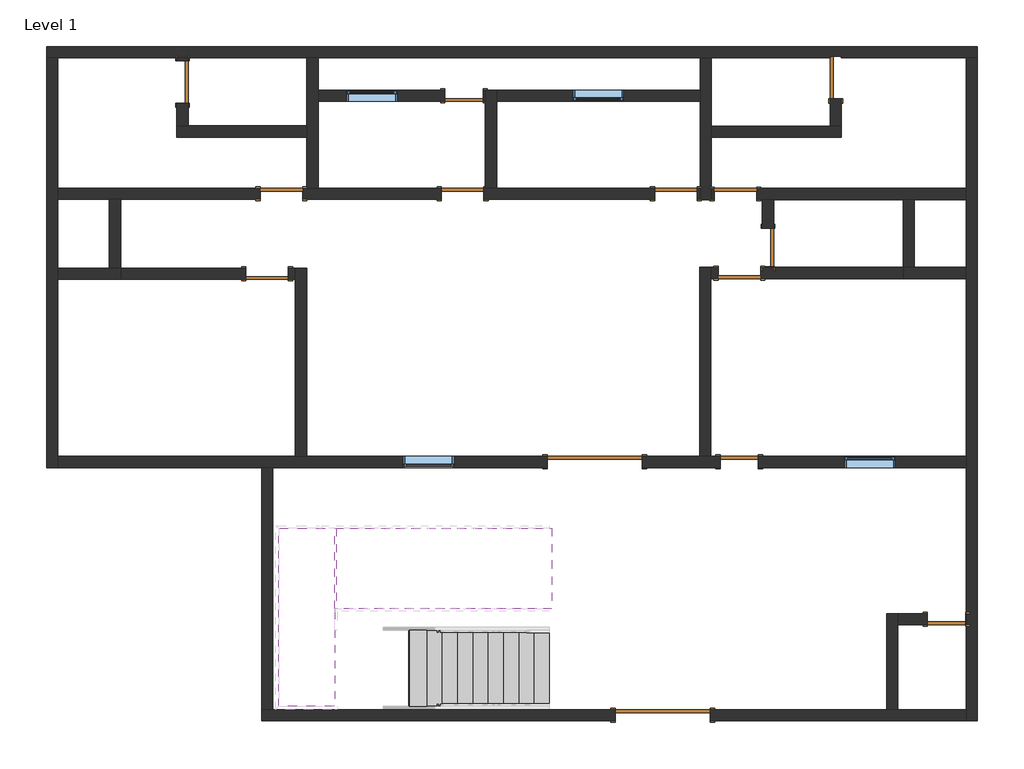
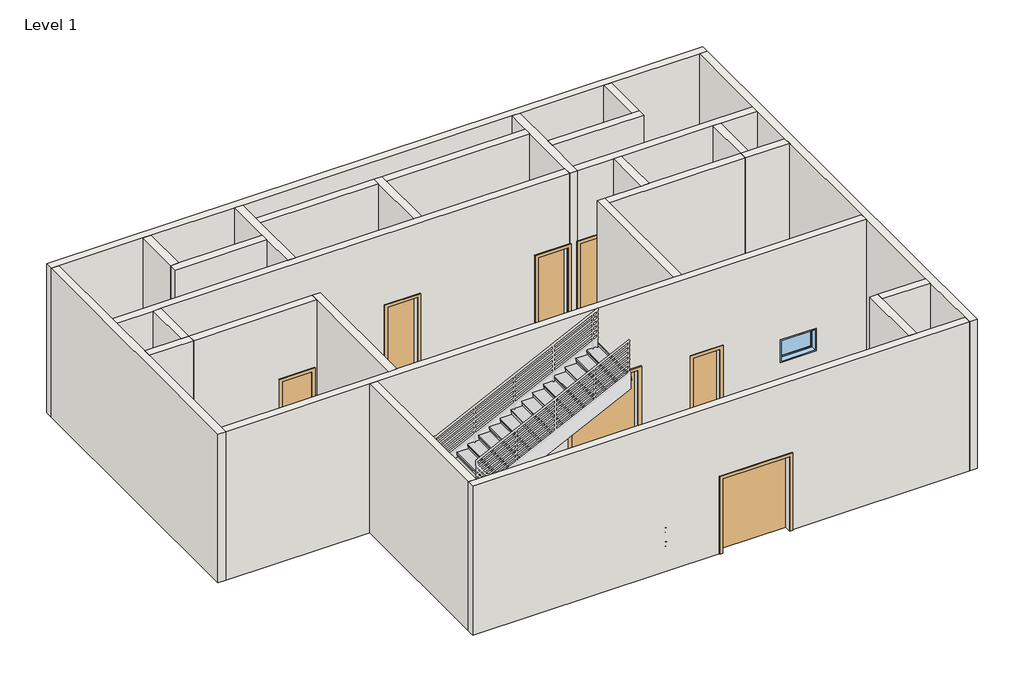
# One storey, part 1 of 4: 28 walls, 14 doors, 4 windows, 2 stair flights, 1 slab.
"""IFC4 building model written with IfcOpenShell, lengths in millimetres."""

from ifc_helpers import new_model, si_unit, frame, origin, origin_with_axes, place, context, project, spatial, polyline, outline, extrude, faceted_brep, transform, mapped, element, save
from components import m_door_double_flush_panel_double_acting_1700_x_2000mm_0a6d9c7f, m_single_flush_0762_x_2032mm_0c256fab, m_single_flush_0762_x_2032mm_7341a4fb, m_single_flush_0762_x_2134mm_f5705a9d, m_single_flush_0762_x_2134mm_85379237, m_single_flush_0762x2022_6401452f, m_single_flush_0762x2022_35973295, non_monolithic_landing_e830aeb0, stair_flight_50mm_tread_25mm_nosing_13mm_riser_e3b9914b, stair_flight_50mm_tread_25mm_nosing_13mm_riser_0c3918f5, m_fixed_0915_x_0610mm_70a843a6

model = new_model("IFC4")

# Units and contexts
model_context = context("Model", 3, world=origin())
ifc_project = project(units=[si_unit("LENGTHUNIT", "METRE", prefix="MILLI")], contexts=[model_context])

# Site, building, storey
site = spatial("IfcSite", under=ifc_project)
building = spatial("IfcBuilding", under=site)
storey = spatial("IfcBuildingStorey", under=building, Name="Level 1", Elevation=0.0)

# Doors
placement = place(None, origin())
m_door_double_flush_panel_double_acting_1700_x_2000mm_shape = m_door_double_flush_panel_double_acting_1700_x_2000mm_0a6d9c7f(model_context)
element("IfcDoor", 1, ObjectType="M_Door-Double-Flush_Panel-Double-Acting : 1700 x 2000mm", at=placement, inside=storey, context=model_context, shape_type="MappedRepresentation", body=[
    mapped(m_door_double_flush_panel_double_acting_1700_x_2000mm_shape, transform((4430.6551601, 3229.9598503, 0.0), x_axis=(1.0, 0.0, 0.0), y_axis=(0.0, 1.0, 0.0), z_axis=(0.0, 0.0, 1.0))),
])
element("IfcDoor", 2, ObjectType="M_Door-Double-Flush_Panel-Double-Acting : 1700 x 2000mm", at=placement, inside=storey, context=model_context, shape_type="MappedRepresentation", body=[
    mapped(m_door_double_flush_panel_double_acting_1700_x_2000mm_shape, transform((5649.8551601, -1313.4901497, 0.0), x_axis=(1.0, 0.0, 0.0), y_axis=(0.0, 1.0, 0.0), z_axis=(0.0, 0.0, 1.0))),
])
m_single_flush_0762_x_2032mm_shape = m_single_flush_0762_x_2032mm_0c256fab(model_context)
element("IfcDoor", 3, ObjectType="M_Single-Flush : 0762 x 2032mm", at=placement, inside=storey, context=model_context, shape_type="MappedRepresentation", body=[
    mapped(m_single_flush_0762_x_2032mm_shape, transform((-1189.0948399, 8036.9098503, 0.0), x_axis=(1.0, 0.0, 0.0), y_axis=(0.0, 1.0, 0.0), z_axis=(0.0, 0.0, 1.0))),
])
element("IfcDoor", 4, ObjectType="M_Single-Flush : 0762 x 2032mm", at=placement, inside=storey, context=model_context, shape_type="MappedRepresentation", body=[
    mapped(m_single_flush_0762_x_2032mm_shape, transform((8750.2551601, 10119.7098503, 0.0), x_axis=(0.0, 1.0, 0.0), y_axis=(-1.0, 0.0, 0.0), z_axis=(0.0, 0.0, 1.0))),
])
element("IfcDoor", 5, ObjectType="M_Single-Flush : 0762 x 2032mm", at=placement, inside=storey, context=model_context, shape_type="MappedRepresentation", body=[
    mapped(m_single_flush_0762_x_2032mm_shape, transform((2062.1051601, 8036.9098503, 0.0), x_axis=(1.0, 0.0, 0.0), y_axis=(0.0, 1.0, 0.0), z_axis=(0.0, 0.0, 1.0))),
])
element("IfcDoor", 6, ObjectType="M_Single-Flush : 0762 x 2032mm", at=placement, inside=storey, context=model_context, shape_type="MappedRepresentation", body=[
    mapped(m_single_flush_0762_x_2032mm_shape, transform((5883.2551601, 8036.9098503, 0.0), x_axis=(1.0, 0.0, 0.0), y_axis=(0.0, 1.0, 0.0), z_axis=(0.0, 0.0, 1.0))),
])
m_single_flush_0762_x_2032mm_2_shape = m_single_flush_0762_x_2032mm_7341a4fb(model_context)
element("IfcDoor", 7, ObjectType="M_Single-Flush : 0762 x 2032mm", at=placement, inside=storey, context=model_context, shape_type="MappedRepresentation", body=[
    mapped(m_single_flush_0762_x_2032mm_2_shape, transform((-2960.7448399, 10043.5098503, 0.0), x_axis=(0.0, 1.0, 0.0), y_axis=(-1.0, 0.0, 0.0), z_axis=(0.0, 0.0, 1.0))),
])
element("IfcDoor", 8, ObjectType="M_Single-Flush : 0762 x 2032mm", at=placement, inside=storey, context=model_context, shape_type="MappedRepresentation", body=[
    mapped(m_single_flush_0762_x_2032mm_2_shape, transform((6950.0551601, 8033.7098503, 0.0), x_axis=(-1.0, 0.0, 0.0), y_axis=(0.0, -1.0, 0.0), z_axis=(0.0, 0.0, 1.0))),
])
m_single_flush_0762_x_2134mm_shape = m_single_flush_0762_x_2134mm_f5705a9d(model_context)
element("IfcDoor", 9, ObjectType="M_Single-Flush : 0762 x 2134mm", at=placement, inside=storey, context=model_context, shape_type="MappedRepresentation", body=[
    mapped(m_single_flush_0762_x_2134mm_shape, transform((-1444.6948399, 6603.4098503, 0.0), x_axis=(1.0, 0.0, 0.0), y_axis=(0.0, 1.0, 0.0), z_axis=(0.0, 0.0, 1.0))),
])
m_single_flush_0762_x_2134mm_2_shape = m_single_flush_0762_x_2134mm_85379237(model_context)
element("IfcDoor", 10, ObjectType="M_Single-Flush : 0762 x 2134mm", at=placement, inside=storey, context=model_context, shape_type="MappedRepresentation", body=[
    mapped(m_single_flush_0762_x_2134mm_2_shape, transform((7021.4551601, 6616.0598503, 0.0), x_axis=(-1.0, 0.0, 0.0), y_axis=(0.0, -1.0, 0.0), z_axis=(0.0, 0.0, 1.0))),
])
m_single_flush_0762x2022_shape = m_single_flush_0762x2022_6401452f(model_context)
element("IfcDoor", 11, ObjectType="M_Single-Flush : 0762X2022", at=placement, inside=storey, context=model_context, shape_type="MappedRepresentation", body=[
    mapped(m_single_flush_0762x2022_shape, transform((2087.5051601, 9792.7098503, 0.0), x_axis=(1.0, 0.0, 0.0), y_axis=(0.0, 1.0, 0.0), z_axis=(0.0, 0.0, 1.0))),
])
element("IfcDoor", 12, ObjectType="M_Single-Flush : 0762X2022", at=placement, inside=storey, context=model_context, shape_type="MappedRepresentation", body=[
    mapped(m_single_flush_0762x2022_shape, transform((10733.0551601, 410.5098503, 0.0), x_axis=(1.0, 0.0, 0.0), y_axis=(0.0, 1.0, 0.0), z_axis=(0.0, 0.0, 1.0))),
])
element("IfcDoor", 13, ObjectType="M_Single-Flush : 0762X2022", at=placement, inside=storey, context=model_context, shape_type="MappedRepresentation", body=[
    mapped(m_single_flush_0762x2022_shape, transform((7021.4551601, 3229.9598503, 0.0), x_axis=(-1.0, 0.0, 0.0), y_axis=(0.0, -1.0, 0.0), z_axis=(0.0, 0.0, 1.0))),
])
m_single_flush_0762x2022_2_shape = m_single_flush_0762x2022_35973295(model_context)
element("IfcDoor", 14, ObjectType="M_Single-Flush : 0762X2022", at=placement, inside=storey, context=model_context, shape_type="MappedRepresentation", body=[
    mapped(m_single_flush_0762x2022_2_shape, transform((7535.8551601, 7073.2598503, 0.0), x_axis=(0.0, -1.0, 0.0), y_axis=(1.0, 0.0, 0.0), z_axis=(0.0, 0.0, 1.0))),
])

# Slab
non_monolithic_landing_shape = non_monolithic_landing_e830aeb0(model_context)
element("IfcSlab", 15, ObjectType="Non-Monolithic Landing", at=placement, inside=storey, context=model_context, shape_type="MappedRepresentation", body=[
    mapped(non_monolithic_landing_shape, transform((0.0, 0.0, 0.0), x_axis=(1.0, 0.0, 0.0), y_axis=(0.0, 1.0, 0.0), z_axis=(0.0, 0.0, 1.0))),
])

# Stair flights
stair_flight_50mm_tread_25mm_nosing_13mm_riser_shape = stair_flight_50mm_tread_25mm_nosing_13mm_riser_e3b9914b(model_context)
element("IfcStairFlight", 16, ObjectType="50mm Tread 25mm Nosing 13mm Riser", at=placement, inside=storey, context=model_context, shape_type="MappedRepresentation", body=[
    mapped(stair_flight_50mm_tread_25mm_nosing_13mm_riser_shape, transform((0.0, 0.0, 0.0), x_axis=(1.0, 0.0, 0.0), y_axis=(0.0, 1.0, 0.0), z_axis=(0.0, 0.0, 1.0))),
])
stair_flight_50mm_tread_25mm_nosing_13mm_riser_2_shape = stair_flight_50mm_tread_25mm_nosing_13mm_riser_0c3918f5(model_context)
element("IfcStairFlight", 17, ObjectType="50mm Tread 25mm Nosing 13mm Riser", at=placement, inside=storey, context=model_context, shape_type="MappedRepresentation", body=[
    mapped(stair_flight_50mm_tread_25mm_nosing_13mm_riser_2_shape, transform((0.0, 0.0, 0.0), x_axis=(1.0, 0.0, 0.0), y_axis=(0.0, 1.0, 0.0), z_axis=(0.0, 0.0, 1.0))),
])

# Walls
element("IfcWall", 18, ObjectType="Generic - 200mm", at=placement, inside=storey, context=model_context, shape_type="Brep", body=[
    faceted_brep([(11290.2551601, 10476.9098503, 4000.0), (11090.2551601, 10476.9098503, 4000.0), (8850.2551601, 10476.9098503, 4000.0), (8650.2551601, 10476.9098503, 4000.0), (6516.6551601, 10476.9098503, 4000.0), (6316.6551601, 10476.9098503, 4000.0), (-530.2948399, 10476.9098503, 4000.0), (-730.2948399, 10476.9098503, 4000.0), (-2860.7448399, 10476.9098503, 4000.0), (-3060.7448399, 10476.9098503, 4000.0), (-5197.5448399, 10476.9098503, 4000.0), (-5397.5448399, 10476.9098503, 4000.0), (-5397.5448399, 10476.9098503, 0.0), (-5197.5448399, 10476.9098503, 0.0), (-3060.7448399, 10476.9098503, 0.0), (-2860.7448399, 10476.9098503, 0.0), (-730.2948399, 10476.9098503, 0.0), (-530.2948399, 10476.9098503, 0.0), (6316.6551601, 10476.9098503, 0.0), (6516.6551601, 10476.9098503, 0.0), (8650.2551601, 10476.9098503, 0.0), (8650.2551601, 10476.9098503, 2032.0), (8850.2551601, 10476.9098503, 2032.0), (8850.2551601, 10476.9098503, 0.0), (11090.2551601, 10476.9098503, 0.0), (11290.2551601, 10476.9098503, 0.0), (11290.2551601, 10676.9098503, 0.0), (-5397.5448399, 10676.9098503, 0.0), (-5397.5448399, 10676.9098503, 4000.0), (11290.2551601, 10676.9098503, 4000.0), (8850.2551601, 10500.7098503, 0.0), (8650.2551601, 10500.7098503, 0.0), (8850.2551601, 10500.7098503, 2032.0), (8650.2551601, 10500.7098503, 2032.0)], [[[0, 1, 2, 3, 4, 5, 6, 7, 8, 9, 10, 11, 12, 13, 14, 15, 16, 17, 18, 19, 20, 21, 22, 23, 24, 25]], [[26, 27, 28, 29]], [[27, 26, 25, 24, 23, 30, 31, 20, 19, 18, 17, 16, 15, 14, 13, 12]], [[11, 10, 9, 8, 7, 6, 5, 4, 3, 2, 1, 0, 29, 28]], [[0, 25, 26, 29]], [[12, 11, 28, 27]], [[32, 30, 23, 22]], [[31, 33, 21, 20]], [[30, 32, 33, 31]], [[33, 32, 22, 21]]]),
])
element("IfcWall", 19, ObjectType="Generic - 200mm", at=placement, inside=storey, context=model_context, shape_type="Brep", body=[
    faceted_brep([(11090.2551601, 10476.9098503, 0.0), (11090.2551601, 8133.7098503, 0.0), (11090.2551601, 7933.7098503, 0.0), (11090.2551601, 6716.0598503, 0.0), (11090.2551601, 6516.0598503, 0.0), (11090.2551601, 3329.9598503, 0.0), (11090.2551601, 3129.9598503, 0.0), (11090.2551601, 510.5098503, 0.0), (11090.2551601, 310.5098503, 0.0), (11090.2551601, -1213.4901497, 0.0), (11090.2551601, -1413.4901497, 0.0), (11090.2551601, -1413.4901497, 4000.0), (11090.2551601, -1213.4901497, 4000.0), (11090.2551601, 310.5098503, 4000.0), (11090.2551601, 510.5098503, 4000.0), (11090.2551601, 3129.9598503, 4000.0), (11090.2551601, 3329.9598503, 4000.0), (11090.2551601, 6516.0598503, 4000.0), (11090.2551601, 6716.0598503, 4000.0), (11090.2551601, 7933.7098503, 4000.0), (11090.2551601, 8133.7098503, 4000.0), (11090.2551601, 10476.9098503, 4000.0), (11290.2551601, 10476.9098503, 0.0), (11290.2551601, 10476.9098503, 4000.0), (11290.2551601, -1413.4901497, 4000.0), (11290.2551601, -1413.4901497, 0.0)], [[[0, 1, 2, 3, 4, 5, 6, 7, 8, 9, 10, 11, 12, 13, 14, 15, 16, 17, 18, 19, 20, 21]], [[22, 23, 24, 25]], [[10, 9, 8, 7, 6, 5, 4, 3, 2, 1, 0, 22, 25]], [[21, 20, 19, 18, 17, 16, 15, 14, 13, 12, 11, 24, 23]], [[0, 21, 23, 22]], [[11, 10, 25, 24]]]),
])
element("IfcWall", 20, ObjectType="Generic - 200mm", at=placement, inside=storey, context=model_context, shape_type="Brep", body=[
    faceted_brep([(-1543.0948399, -1213.4901497, 4000.0), (-1343.0948399, -1213.4901497, 4000.0), (9664.6551601, -1213.4901497, 4000.0), (9864.6551601, -1213.4901497, 4000.0), (11090.2551601, -1213.4901497, 4000.0), (11090.2551601, -1213.4901497, 0.0), (9864.6551601, -1213.4901497, 0.0), (9664.6551601, -1213.4901497, 0.0), (6499.8551601, -1213.4901497, 0.0), (6499.8551601, -1213.4901497, 2000.0), (4799.8551601, -1213.4901497, 2000.0), (4799.8551601, -1213.4901497, 0.0), (-1343.0948399, -1213.4901497, 0.0), (-1543.0948399, -1213.4901497, 0.0), (11090.2551601, -1413.4901497, 4000.0), (-1543.0948399, -1413.4901497, 4000.0), (-1543.0948399, -1413.4901497, 0.0), (4799.8551601, -1413.4901497, 0.0), (4799.8551601, -1413.4901497, 2000.0), (6499.8551601, -1413.4901497, 2000.0), (6499.8551601, -1413.4901497, 0.0), (11090.2551601, -1413.4901497, 0.0)], [[[0, 1, 2, 3, 4, 5, 6, 7, 8, 9, 10, 11, 12, 13]], [[14, 15, 16, 17, 18, 19, 20, 21]], [[5, 21, 20, 8, 7, 6]], [[16, 13, 12, 11, 17]], [[4, 3, 2, 1, 0, 15, 14]], [[5, 4, 14, 21]], [[0, 13, 16, 15]], [[19, 9, 8, 20]], [[9, 19, 18, 10]], [[10, 18, 17, 11]]]),
])
element("IfcWall", 21, ObjectType="Generic - 200mm", at=placement, inside=storey, context=model_context, shape_type="Brep", body=[
    faceted_brep([(-5197.5448399, 3129.9598503, 0.0), (-5197.5448399, 3329.9598503, 0.0), (-5197.5448399, 6503.4098503, 0.0), (-5197.5448399, 6703.4098503, 0.0), (-5197.5448399, 7936.9098503, 0.0), (-5197.5448399, 8136.9098503, 0.0), (-5197.5448399, 10476.9098503, 0.0), (-5197.5448399, 10476.9098503, 4000.0), (-5197.5448399, 8136.9098503, 4000.0), (-5197.5448399, 7936.9098503, 4000.0), (-5197.5448399, 6703.4098503, 4000.0), (-5197.5448399, 6503.4098503, 4000.0), (-5197.5448399, 3329.9598503, 4000.0), (-5197.5448399, 3129.9598503, 4000.0), (-5397.5448399, 3129.9598503, 0.0), (-5397.5448399, 3129.9598503, 4000.0), (-5397.5448399, 10476.9098503, 4000.0), (-5397.5448399, 10476.9098503, 0.0)], [[[0, 1, 2, 3, 4, 5, 6, 7, 8, 9, 10, 11, 12, 13]], [[14, 15, 16, 17]], [[6, 5, 4, 3, 2, 1, 0, 14, 17]], [[13, 12, 11, 10, 9, 8, 7, 16, 15]], [[7, 6, 17, 16]], [[0, 13, 15, 14]]]),
])
element("IfcWall", 22, ObjectType="Generic - 200mm", at=placement, inside=storey, context=model_context, shape_type="Brep", body=[
    faceted_brep([(-530.2948399, 8136.9098503, 0.0), (-530.2948399, 9692.7098503, 0.0), (-530.2948399, 9892.7098503, 0.0), (-530.2948399, 10476.9098503, 0.0), (-530.2948399, 10476.9098503, 4000.0), (-530.2948399, 9892.7098503, 4000.0), (-530.2948399, 9692.7098503, 4000.0), (-530.2948399, 8136.9098503, 4000.0), (-730.2948399, 8136.9098503, 0.0), (-730.2948399, 8136.9098503, 4000.0), (-730.2948399, 9052.9098503, 4000.0), (-730.2948399, 9252.9098503, 4000.0), (-730.2948399, 10476.9098503, 4000.0), (-730.2948399, 10476.9098503, 0.0), (-730.2948399, 9252.9098503, 0.0), (-730.2948399, 9052.9098503, 0.0)], [[[0, 1, 2, 3, 4, 5, 6, 7]], [[8, 9, 10, 11, 12, 13, 14, 15]], [[3, 2, 1, 0, 8, 15, 14, 13]], [[7, 6, 5, 4, 12, 11, 10, 9]], [[4, 3, 13, 12]], [[0, 7, 9, 8]]]),
])
element("IfcWall", 23, ObjectType="Generic - 200mm", at=placement, inside=storey, context=model_context, shape_type="Brep", body=[
    faceted_brep([(6264.2551601, 7936.9098503, 2032.0), (6264.2551601, 7936.9098503, 0.0), (6316.6551601, 7936.9098503, 0.0), (6316.6551601, 7936.9098503, 4000.0), (-4070.4448399, 7936.9098503, 4000.0), (-4270.4448399, 7936.9098503, 4000.0), (-5197.5448399, 7936.9098503, 4000.0), (-5197.5448399, 7936.9098503, 0.0), (-4270.4448399, 7936.9098503, 0.0), (-4070.4448399, 7936.9098503, 0.0), (-1570.0948399, 7936.9098503, 0.0), (-1570.0948399, 7936.9098503, 2032.0), (-808.0948399, 7936.9098503, 2032.0), (-808.0948399, 7936.9098503, 0.0), (1681.1051601, 7936.9098503, 0.0), (1681.1051601, 7936.9098503, 2032.0), (2443.1051601, 7936.9098503, 2032.0), (2443.1051601, 7936.9098503, 0.0), (5502.2551601, 7936.9098503, 0.0), (5502.2551601, 7936.9098503, 2032.0), (6316.6551601, 8136.9098503, 0.0), (6264.2551601, 8136.9098503, 0.0), (6264.2551601, 8136.9098503, 2032.0), (5502.2551601, 8136.9098503, 2032.0), (5502.2551601, 8136.9098503, 0.0), (2670.1051601, 8136.9098503, 0.0), (2470.1051601, 8136.9098503, 0.0), (2443.1051601, 8136.9098503, 0.0), (2443.1051601, 8136.9098503, 2032.0), (1681.1051601, 8136.9098503, 2032.0), (1681.1051601, 8136.9098503, 0.0), (-530.2948399, 8136.9098503, 0.0), (-730.2948399, 8136.9098503, 0.0), (-808.0948399, 8136.9098503, 0.0), (-808.0948399, 8136.9098503, 2032.0), (-1570.0948399, 8136.9098503, 2032.0), (-1570.0948399, 8136.9098503, 0.0), (-5197.5448399, 8136.9098503, 0.0), (-5197.5448399, 8136.9098503, 4000.0), (-730.2948399, 8136.9098503, 4000.0), (-530.2948399, 8136.9098503, 4000.0), (2470.1051601, 8136.9098503, 4000.0), (2670.1051601, 8136.9098503, 4000.0), (6316.6551601, 8136.9098503, 4000.0)], [[[0, 1, 2, 3, 4, 5, 6, 7, 8, 9, 10, 11, 12, 13, 14, 15, 16, 17, 18, 19]], [[20, 21, 22, 23, 24, 25, 26, 27, 28, 29, 30, 31, 32, 33, 34, 35, 36, 37, 38, 39, 40, 41, 42, 43]], [[14, 13, 33, 32, 31, 30]], [[18, 17, 27, 26, 25, 24]], [[2, 1, 21, 20]], [[10, 9, 8, 7, 37, 36]], [[6, 5, 4, 3, 43, 42, 41, 40, 39, 38]], [[7, 6, 38, 37]], [[34, 33, 13, 12]], [[35, 34, 12, 11]], [[36, 35, 11, 10]], [[3, 2, 20, 43]], [[28, 27, 17, 16]], [[29, 28, 16, 15]], [[30, 29, 15, 14]], [[22, 21, 1, 0]], [[23, 22, 0, 19]], [[24, 23, 19, 18]]]),
])
element("IfcWall", 24, ObjectType="Generic - 200mm", at=placement, inside=storey, context=model_context, shape_type="Brep", body=[
    faceted_brep([(-730.2948399, 9252.9098503, 0.0), (-2860.7448399, 9252.9098503, 0.0), (-3060.7448399, 9252.9098503, 0.0), (-3060.7448399, 9252.9098503, 4000.0), (-2860.7448399, 9252.9098503, 4000.0), (-730.2948399, 9252.9098503, 4000.0), (-730.2948399, 9052.9098503, 0.0), (-730.2948399, 9052.9098503, 4000.0), (-3060.7448399, 9052.9098503, 4000.0), (-3060.7448399, 9052.9098503, 0.0)], [[[0, 1, 2, 3, 4, 5]], [[6, 7, 8, 9]], [[2, 1, 0, 6, 9]], [[5, 4, 3, 8, 7]], [[0, 5, 7, 6]], [[3, 2, 9, 8]]]),
])
element("IfcWall", 25, ObjectType="Generic - 200mm", at=placement, inside=storey, context=model_context, shape_type="SweptSolid", body=[
    extrude(outline(polyline([(10476.9098503, 0.0), (10424.5098503, 0.0), (10424.5098503, 2032.0), (9662.5098503, 2032.0), (9662.5098503, 0.0), (9252.9098503, 0.0), (9252.9098503, 4000.0), (10476.9098503, 4000.0), (10476.9098503, 0.0)])), frame((-3060.7448399, 0.0, 0.0), z_axis=(1.0, 0.0, 0.0), x_axis=(0.0, 1.0, 0.0)), (0.0, 0.0, 1.0), 200.0),
])
element("IfcWall", 26, ObjectType="Generic - 200mm", at=placement, inside=storey, context=model_context, shape_type="Brep", body=[
    faceted_brep([(6316.6551601, 10476.9098503, 0.0), (6316.6551601, 9892.7098503, 0.0), (6316.6551601, 9692.7098503, 0.0), (6316.6551601, 8136.9098503, 0.0), (6316.6551601, 7936.9098503, 0.0), (6316.6551601, 7933.7098503, 0.0), (6316.6551601, 7933.7098503, 4000.0), (6316.6551601, 7936.9098503, 4000.0), (6316.6551601, 8136.9098503, 4000.0), (6316.6551601, 9692.7098503, 4000.0), (6316.6551601, 9892.7098503, 4000.0), (6316.6551601, 10476.9098503, 4000.0), (6516.6551601, 10476.9098503, 0.0), (6516.6551601, 10476.9098503, 4000.0), (6516.6551601, 9248.1598503, 4000.0), (6516.6551601, 9048.1598503, 4000.0), (6516.6551601, 8133.7098503, 4000.0), (6516.6551601, 7933.7098503, 4000.0), (6516.6551601, 7933.7098503, 0.0), (6516.6551601, 8133.7098503, 0.0), (6516.6551601, 9048.1598503, 0.0), (6516.6551601, 9248.1598503, 0.0)], [[[0, 1, 2, 3, 4, 5, 6, 7, 8, 9, 10, 11]], [[12, 13, 14, 15, 16, 17, 18, 19, 20, 21]], [[5, 4, 3, 2, 1, 0, 12, 21, 20, 19, 18]], [[11, 10, 9, 8, 7, 6, 17, 16, 15, 14, 13]], [[0, 11, 13, 12]], [[6, 5, 18, 17]]]),
])
element("IfcWall", 27, ObjectType="Generic - 200mm", at=placement, inside=storey, context=model_context, shape_type="Brep", body=[
    faceted_brep([(6516.6551601, 7933.7098503, 0.0), (6569.0551601, 7933.7098503, 0.0), (6569.0551601, 7933.7098503, 2032.0), (7331.0551601, 7933.7098503, 2032.0), (7331.0551601, 7933.7098503, 0.0), (7435.8551601, 7933.7098503, 0.0), (7635.8551601, 7933.7098503, 0.0), (9959.9551601, 7933.7098503, 0.0), (10159.9551601, 7933.7098503, 0.0), (11090.2551601, 7933.7098503, 0.0), (11090.2551601, 7933.7098503, 4000.0), (10159.9551601, 7933.7098503, 4000.0), (9959.9551601, 7933.7098503, 4000.0), (7635.8551601, 7933.7098503, 4000.0), (7435.8551601, 7933.7098503, 4000.0), (6516.6551601, 7933.7098503, 4000.0), (6569.0551601, 8133.7098503, 2032.0), (6569.0551601, 8133.7098503, 0.0), (6516.6551601, 8133.7098503, 0.0), (6516.6551601, 8133.7098503, 4000.0), (11090.2551601, 8133.7098503, 4000.0), (11090.2551601, 8133.7098503, 0.0), (7331.0551601, 8133.7098503, 0.0), (7331.0551601, 8133.7098503, 2032.0)], [[[0, 1, 2, 3, 4, 5, 6, 7, 8, 9, 10, 11, 12, 13, 14, 15]], [[16, 17, 18, 19, 20, 21, 22, 23]], [[22, 21, 9, 8, 7, 6, 5, 4]], [[18, 17, 1, 0]], [[15, 14, 13, 12, 11, 10, 20, 19]], [[0, 15, 19, 18]], [[10, 9, 21, 20]], [[2, 1, 17, 16]], [[3, 2, 16, 23]], [[4, 3, 23, 22]]]),
])
element("IfcWall", 28, ObjectType="Generic - 200mm", at=placement, inside=storey, context=model_context, shape_type="Brep", body=[
    faceted_brep([(6516.6551601, 9048.1598503, 0.0), (8850.2551601, 9048.1598503, 0.0), (8850.2551601, 9048.1598503, 4000.0), (6516.6551601, 9048.1598503, 4000.0), (6516.6551601, 9248.1598503, 0.0), (6516.6551601, 9248.1598503, 4000.0), (8650.2551601, 9248.1598503, 4000.0), (8850.2551601, 9248.1598503, 4000.0), (8850.2551601, 9248.1598503, 0.0), (8650.2551601, 9248.1598503, 0.0)], [[[0, 1, 2, 3]], [[4, 5, 6, 7, 8, 9]], [[1, 0, 4, 9, 8]], [[3, 2, 7, 6, 5]], [[0, 3, 5, 4]], [[2, 1, 8, 7]]]),
])
element("IfcWall", 29, ObjectType="Generic - 200mm", at=placement, inside=storey, context=model_context, shape_type="SweptSolid", body=[
    extrude(outline(polyline([(9248.1598503, 4000.0), (10476.9098503, 4000.0), (10476.9098503, 2032.0), (9738.7098503, 2032.0), (9738.7098503, 0.0), (9248.1598503, 0.0), (9248.1598503, 4000.0)])), frame((8650.2551601, 0.0, 0.0), z_axis=(1.0, 0.0, 0.0), x_axis=(0.0, 1.0, 0.0)), (0.0, 0.0, 1.0), 200.0),
])
element("IfcWall", 30, ObjectType="Generic - 200mm", at=placement, inside=storey, context=model_context, shape_type="Brep", body=[
    faceted_brep([(2670.1051601, 8136.9098503, 0.0), (2670.1051601, 9692.7098503, 0.0), (2670.1051601, 9892.7098503, 0.0), (2670.1051601, 9892.7098503, 4000.0), (2670.1051601, 9692.7098503, 4000.0), (2670.1051601, 8136.9098503, 4000.0), (2470.1051601, 8136.9098503, 0.0), (2470.1051601, 8136.9098503, 4000.0), (2470.1051601, 9692.7098503, 4000.0), (2470.1051601, 9892.7098503, 4000.0), (2470.1051601, 9892.7098503, 0.0), (2470.1051601, 9692.7098503, 0.0)], [[[0, 1, 2, 3, 4, 5]], [[6, 7, 8, 9, 10, 11]], [[2, 1, 0, 6, 11, 10]], [[5, 4, 3, 9, 8, 7]], [[0, 5, 7, 6]], [[3, 2, 10, 9]]]),
])
element("IfcWall", 31, ObjectType="Generic - 200mm", at=placement, inside=storey, context=model_context, shape_type="SweptSolid", body=[
    extrude(outline(polyline([(1828.8, 2430.4051601), (0.0, 2430.4051601), (0.0, 2470.1051601), (4000.0, 2470.1051601), (4000.0, -530.2948399), (0.0, -530.2948399), (0.0, 1744.6051601), (1828.8, 1744.6051601), (1828.8, 2430.4051601)]), holes=[polyline([(915.0, -20.9948399), (1525.0, -20.9948399), (1525.0, 894.0051601), (915.0, 894.0051601), (915.0, -20.9948399)])]), frame((0.0, 9692.7098503, 0.0), z_axis=(0.0, 1.0, 0.0), x_axis=(0.0, 0.0, 1.0)), (0.0, 0.0, 1.0), 200.0),
])
element("IfcWall", 32, ObjectType="Generic - 200mm", at=placement, inside=storey, context=model_context, shape_type="SweptSolid", body=[
    extrude(outline(polyline([(0.0, 2670.1051601), (0.0, 6316.6551601), (4000.0, 6316.6551601), (4000.0, 2670.1051601), (0.0, 2670.1051601)]), holes=[polyline([(915.0, 4950.8801601), (915.0, 4035.8801601), (1525.0, 4035.8801601), (1525.0, 4950.8801601), (915.0, 4950.8801601)])]), frame((0.0, 9692.7098503, 0.0), z_axis=(0.0, 1.0, 0.0), x_axis=(0.0, 0.0, 1.0)), (0.0, 0.0, 1.0), 200.0),
])
element("IfcWall", 33, ObjectType="Generic - 200mm", at=placement, inside=storey, context=model_context, shape_type="Brep", body=[
    faceted_brep([(-5197.5448399, 6503.4098503, 0.0), (-4070.4448399, 6503.4098503, 0.0), (-4070.4448399, 6503.4098503, 4000.0), (-5197.5448399, 6503.4098503, 4000.0), (-5197.5448399, 6703.4098503, 0.0), (-5197.5448399, 6703.4098503, 4000.0), (-4270.4448399, 6703.4098503, 4000.0), (-4070.4448399, 6703.4098503, 4000.0), (-4070.4448399, 6703.4098503, 0.0), (-4270.4448399, 6703.4098503, 0.0)], [[[0, 1, 2, 3]], [[4, 5, 6, 7, 8, 9]], [[1, 0, 4, 9, 8]], [[3, 2, 7, 6, 5]], [[0, 3, 5, 4]], [[2, 1, 8, 7]]]),
])
element("IfcWall", 34, ObjectType="Generic - 200mm", at=placement, inside=storey, context=model_context, shape_type="SweptSolid", body=[
    extrude(outline(polyline([(-4070.4448399, 7936.9098503), (-4070.4448399, 6703.4098503), (-4270.4448399, 6703.4098503), (-4270.4448399, 7936.9098503), (-4070.4448399, 7936.9098503)])), origin_with_axes(), (0.0, 0.0, 1.0), 4000.0),
])
element("IfcWall", 35, ObjectType="Generic - 200mm", at=placement, inside=storey, context=model_context, shape_type="Brep", body=[
    faceted_brep([(11090.2551601, 6716.0598503, 0.0), (10159.9551601, 6716.0598503, 0.0), (9959.9551601, 6716.0598503, 0.0), (9959.9551601, 6716.0598503, 4000.0), (10159.9551601, 6716.0598503, 4000.0), (11090.2551601, 6716.0598503, 4000.0), (11090.2551601, 6516.0598503, 0.0), (11090.2551601, 6516.0598503, 4000.0), (9959.9551601, 6516.0598503, 4000.0), (9959.9551601, 6516.0598503, 0.0)], [[[0, 1, 2, 3, 4, 5]], [[6, 7, 8, 9]], [[2, 1, 0, 6, 9]], [[5, 4, 3, 8, 7]], [[0, 5, 7, 6]], [[3, 2, 9, 8]]]),
])
element("IfcWall", 36, ObjectType="Generic - 200mm", at=placement, inside=storey, context=model_context, shape_type="SweptSolid", body=[
    extrude(outline(polyline([(10159.9551601, 7933.7098503), (10159.9551601, 6716.0598503), (9959.9551601, 6716.0598503), (9959.9551601, 7933.7098503), (10159.9551601, 7933.7098503)])), origin_with_axes(), (0.0, 0.0, 1.0), 4000.0),
])
element("IfcWall", 37, ObjectType="Generic - 200mm", at=placement, inside=storey, context=model_context, shape_type="Brep", body=[
    faceted_brep([(6678.5551601, 3329.9598503, 1828.8), (6678.5551601, 3329.9598503, 0.0), (6511.8551601, 3329.9598503, 0.0), (6311.8551601, 3329.9598503, 0.0), (5280.6551601, 3329.9598503, 0.0), (5280.6551601, 3329.9598503, 2000.0), (3580.6551601, 3329.9598503, 2000.0), (3580.6551601, 3329.9598503, 0.0), (-735.0948399, 3329.9598503, 0.0), (-935.0948399, 3329.9598503, 0.0), (-5197.5448399, 3329.9598503, 0.0), (-5197.5448399, 3329.9598503, 4000.0), (-935.0948399, 3329.9598503, 4000.0), (-735.0948399, 3329.9598503, 4000.0), (6311.8551601, 3329.9598503, 4000.0), (6511.8551601, 3329.9598503, 4000.0), (11090.2551601, 3329.9598503, 4000.0), (11090.2551601, 3329.9598503, 0.0), (7364.3551601, 3329.9598503, 0.0), (7364.3551601, 3329.9598503, 1828.8), (1908.4051601, 3329.9598503, 915.0), (1908.4051601, 3329.9598503, 1525.0), (993.4051601, 3329.9598503, 1525.0), (993.4051601, 3329.9598503, 915.0), (8903.9551601, 3329.9598503, 915.0), (9818.9551601, 3329.9598503, 915.0), (9818.9551601, 3329.9598503, 1525.0), (8903.9551601, 3329.9598503, 1525.0), (5280.6551601, 3129.9598503, 0.0), (6678.5551601, 3129.9598503, 0.0), (6678.5551601, 3129.9598503, 1828.8), (7364.3551601, 3129.9598503, 1828.8), (7364.3551601, 3129.9598503, 0.0), (11090.2551601, 3129.9598503, 0.0), (11090.2551601, 3129.9598503, 4000.0), (-1343.0948399, 3129.9598503, 4000.0), (-1543.0948399, 3129.9598503, 4000.0), (-5197.5448399, 3129.9598503, 4000.0), (-5197.5448399, 3129.9598503, 0.0), (-1543.0948399, 3129.9598503, 0.0), (-1343.0948399, 3129.9598503, 0.0), (3580.6551601, 3129.9598503, 0.0), (3580.6551601, 3129.9598503, 2000.0), (5280.6551601, 3129.9598503, 2000.0), (1908.4051601, 3129.9598503, 915.0), (993.4051601, 3129.9598503, 915.0), (993.4051601, 3129.9598503, 1525.0), (1908.4051601, 3129.9598503, 1525.0), (8903.9551601, 3129.9598503, 915.0), (8903.9551601, 3129.9598503, 1525.0), (9818.9551601, 3129.9598503, 1525.0), (9818.9551601, 3129.9598503, 915.0)], [[[0, 1, 2, 3, 4, 5, 6, 7, 8, 9, 10, 11, 12, 13, 14, 15, 16, 17, 18, 19], [20, 21, 22, 23], [24, 25, 26, 27]], [[28, 29, 30, 31, 32, 33, 34, 35, 36, 37, 38, 39, 40, 41, 42, 43], [44, 45, 46, 47], [48, 49, 50, 51]], [[38, 10, 9, 8, 7, 41, 40, 39]], [[18, 17, 33, 32]], [[4, 3, 2, 1, 29, 28]], [[16, 15, 14, 13, 12, 11, 37, 36, 35, 34]], [[17, 16, 34, 33]], [[43, 5, 4, 28]], [[5, 43, 42, 6]], [[6, 42, 41, 7]], [[11, 10, 38, 37]], [[21, 20, 44, 47]], [[22, 21, 47, 46]], [[23, 22, 46, 45]], [[20, 23, 45, 44]], [[49, 48, 24, 27]], [[50, 49, 27, 26]], [[51, 50, 26, 25]], [[48, 51, 25, 24]], [[30, 29, 1, 0]], [[31, 30, 0, 19]], [[32, 31, 19, 18]]]),
])
element("IfcWall", 38, ObjectType="Generic - 200mm", at=placement, inside=storey, context=model_context, shape_type="Brep", body=[
    faceted_brep([(6511.8551601, 3329.9598503, 0.0), (6511.8551601, 6516.0598503, 0.0), (6511.8551601, 6716.0598503, 0.0), (6511.8551601, 6716.0598503, 4000.0), (6511.8551601, 6516.0598503, 4000.0), (6511.8551601, 3329.9598503, 4000.0), (6311.8551601, 3329.9598503, 0.0), (6311.8551601, 3329.9598503, 4000.0), (6311.8551601, 6716.0598503, 4000.0), (6311.8551601, 6716.0598503, 0.0)], [[[0, 1, 2, 3, 4, 5]], [[6, 7, 8, 9]], [[2, 1, 0, 6, 9]], [[5, 4, 3, 8, 7]], [[0, 5, 7, 6]], [[3, 2, 9, 8]]]),
])
element("IfcWall", 39, ObjectType="Generic - 200mm", at=placement, inside=storey, context=model_context, shape_type="Brep", body=[
    faceted_brep([(6511.8551601, 6516.0598503, 0.0), (6640.4551601, 6516.0598503, 0.0), (6640.4551601, 6516.0598503, 2134.0), (7402.4551601, 6516.0598503, 2134.0), (7402.4551601, 6516.0598503, 0.0), (9959.9551601, 6516.0598503, 0.0), (9959.9551601, 6516.0598503, 4000.0), (6511.8551601, 6516.0598503, 4000.0), (6640.4551601, 6716.0598503, 2134.0), (6640.4551601, 6716.0598503, 0.0), (6511.8551601, 6716.0598503, 0.0), (6511.8551601, 6716.0598503, 4000.0), (7435.8551601, 6716.0598503, 4000.0), (7635.8551601, 6716.0598503, 4000.0), (9959.9551601, 6716.0598503, 4000.0), (9959.9551601, 6716.0598503, 0.0), (7635.8551601, 6716.0598503, 0.0), (7435.8551601, 6716.0598503, 0.0), (7402.4551601, 6716.0598503, 0.0), (7402.4551601, 6716.0598503, 2134.0)], [[[0, 1, 2, 3, 4, 5, 6, 7]], [[8, 9, 10, 11, 12, 13, 14, 15, 16, 17, 18, 19]], [[10, 9, 1, 0]], [[18, 17, 16, 15, 5, 4]], [[7, 6, 14, 13, 12, 11]], [[0, 7, 11, 10]], [[6, 5, 15, 14]], [[2, 1, 9, 8]], [[3, 2, 8, 19]], [[4, 3, 19, 18]]]),
])
element("IfcWall", 40, ObjectType="Generic - 200mm", at=placement, inside=storey, context=model_context, shape_type="Brep", body=[
    faceted_brep([(-735.0948399, 3329.9598503, 0.0), (-735.0948399, 6703.4098503, 0.0), (-735.0948399, 6703.4098503, 4000.0), (-735.0948399, 3329.9598503, 4000.0), (-935.0948399, 3329.9598503, 0.0), (-935.0948399, 3329.9598503, 4000.0), (-935.0948399, 6503.4098503, 4000.0), (-935.0948399, 6703.4098503, 4000.0), (-935.0948399, 6703.4098503, 0.0), (-935.0948399, 6503.4098503, 0.0)], [[[0, 1, 2, 3]], [[4, 5, 6, 7, 8, 9]], [[1, 0, 4, 9, 8]], [[3, 2, 7, 6, 5]], [[0, 3, 5, 4]], [[2, 1, 8, 7]]]),
])
element("IfcWall", 41, ObjectType="Generic - 200mm", at=placement, inside=storey, context=model_context, shape_type="SweptSolid", body=[
    extrude(outline(polyline([(2134.0, -1063.6948399), (0.0, -1063.6948399), (0.0, -935.0948399), (4000.0, -935.0948399), (4000.0, -4070.4448399), (0.0, -4070.4448399), (0.0, -1825.6948399), (2134.0, -1825.6948399), (2134.0, -1063.6948399)])), frame((0.0, 6503.4098503, 0.0), z_axis=(0.0, 1.0, 0.0), x_axis=(0.0, 0.0, 1.0)), (0.0, 0.0, 1.0), 200.0),
])
element("IfcWall", 42, ObjectType="Generic - 200mm", at=placement, inside=storey, context=model_context, shape_type="SweptSolid", body=[
    extrude(outline(polyline([(6730.3598503, 1828.8), (6730.3598503, 0.0), (6716.0598503, 0.0), (6716.0598503, 4000.0), (7933.7098503, 4000.0), (7933.7098503, 0.0), (7416.1598503, 0.0), (7416.1598503, 1828.8), (6730.3598503, 1828.8)])), frame((7435.8551601, 0.0, 0.0), z_axis=(1.0, 0.0, 0.0), x_axis=(0.0, 1.0, 0.0)), (0.0, 0.0, 1.0), 200.0),
])
element("IfcWall", 43, ObjectType="Generic - 200mm", at=placement, inside=storey, context=model_context, shape_type="Brep", body=[
    faceted_brep([(9864.6551601, -1213.4901497, 0.0), (9864.6551601, 310.5098503, 0.0), (9864.6551601, 510.5098503, 0.0), (9864.6551601, 510.5098503, 4000.0), (9864.6551601, 310.5098503, 4000.0), (9864.6551601, -1213.4901497, 4000.0), (9664.6551601, -1213.4901497, 0.0), (9664.6551601, -1213.4901497, 4000.0), (9664.6551601, 510.5098503, 4000.0), (9664.6551601, 510.5098503, 0.0)], [[[0, 1, 2, 3, 4, 5]], [[6, 7, 8, 9]], [[2, 1, 0, 6, 9]], [[5, 4, 3, 8, 7]], [[0, 5, 7, 6]], [[3, 2, 9, 8]]]),
])
element("IfcWall", 44, ObjectType="Generic - 200mm", at=placement, inside=storey, context=model_context, shape_type="SweptSolid", body=[
    extrude(outline(polyline([(1828.8, 11075.9551601), (0.0, 11075.9551601), (0.0, 11090.2551601), (4000.0, 11090.2551601), (4000.0, 9864.6551601), (0.0, 9864.6551601), (0.0, 10390.1551601), (1828.8, 10390.1551601), (1828.8, 11075.9551601)])), frame((0.0, 310.5098503, 0.0), z_axis=(0.0, 1.0, 0.0), x_axis=(0.0, 0.0, 1.0)), (0.0, 0.0, 1.0), 200.0),
])
element("IfcWall", 45, ObjectType="Generic - 200mm", at=placement, inside=storey, context=model_context, shape_type="SweptSolid", body=[
    extrude(outline(polyline([(-1543.0948399, -1213.4901497), (-1543.0948399, 3129.9598503), (-1343.0948399, 3129.9598503), (-1343.0948399, -1213.4901497), (-1543.0948399, -1213.4901497)])), origin_with_axes(), (0.0, 0.0, 1.0), 4000.0),
])

# Windows
m_fixed_0915_x_0610mm_shape = m_fixed_0915_x_0610mm_70a843a6(model_context)
element("IfcWindow", 46, ObjectType="M_Fixed : 0915 x 0610mm", at=placement, inside=storey, context=model_context, shape_type="MappedRepresentation", body=[
    mapped(m_fixed_0915_x_0610mm_shape, transform((436.5051601, 9779.7098503, 0.0), x_axis=(1.0, 0.0, 0.0), y_axis=(0.0, 1.0, 0.0), z_axis=(0.0, 0.0, 1.0))),
])
element("IfcWindow", 47, ObjectType="M_Fixed : 0915 x 0610mm", at=placement, inside=storey, context=model_context, shape_type="MappedRepresentation", body=[
    mapped(m_fixed_0915_x_0610mm_shape, transform((4493.3801601, 9805.7098503, 0.0), x_axis=(-1.0, 0.0, 0.0), y_axis=(0.0, -1.0, 0.0), z_axis=(0.0, 0.0, 1.0))),
])
element("IfcWindow", 48, ObjectType="M_Fixed : 0915 x 0610mm", at=placement, inside=storey, context=model_context, shape_type="MappedRepresentation", body=[
    mapped(m_fixed_0915_x_0610mm_shape, transform((1450.9051601, 3242.9598503, 0.0), x_axis=(-1.0, 0.0, 0.0), y_axis=(0.0, -1.0, 0.0), z_axis=(0.0, 0.0, 1.0))),
])
element("IfcWindow", 49, ObjectType="M_Fixed : 0915 x 0610mm", at=placement, inside=storey, context=model_context, shape_type="MappedRepresentation", body=[
    mapped(m_fixed_0915_x_0610mm_shape, transform((9361.4551601, 3216.9598503, 0.0), x_axis=(1.0, 0.0, 0.0), y_axis=(0.0, 1.0, 0.0), z_axis=(0.0, 0.0, 1.0))),
])

save(model, "model.ifc")

# Revit data of these elements
# Type "M_Door-Double-Flush_Panel-Double-Acting : 1700 x 2000mm"
#   Type Mark = "23"
#   Construction Type Id = "DOOR"
#   Assembly Code = "C1020"
#   Analytic Construction = "Wooden"
#   W = 2' - 9.46457"
#   Thickness = 0' - 1.9685"
#   Thermal Resistance (R) = 0.455703 (m²·K)/W
#   Swing Angle [instance default] = 90.00°
#   Heat Transfer Coefficient (U) = 2.19465 W/(m²·K)
#   Height = 6' - 6.74016"
#   Trim Projection Ext. = 0' - 0.98425"
#   Trim Projection Int. = 0' - 0.98425"
#   Trim Width Ext. = 0' - 3.14961"
#   Trim Width Int. = 0' - 3.14961"
#   Width = 5' - 6.92913"
#   Define Thermal Properties by = 1
#   Panel Material = Wood - Birch - Solid Stained Light Low Gloss
#   Trim Material = Paint - Sienna
#   Visual Light Transmittance = 0
#   Solar Heat Gain Coefficient = 0
#   Function = (empty or 0)
#   Wall Closure = (empty or 0)
# Type "M_Single-Flush : 0762 x 2032mm"
#   Type Mark = "19"
#   Thickness = 0' - 2.00787"
#   Height = 6' - 8"
#   Trim Projection Ext = 0' - 0.98425"
#   Trim Projection Int = 0' - 0.98425"
#   Trim Width = 0' - 2.99213"
#   Width = 2' - 6"
#   Door Material = Door - Panel
#   Frame Material = Door - Frame
#   Function = (empty or 0)
#   Wall Closure = (empty or 0)
# Type "M_Single-Flush : 0762 x 2134mm"
#   Type Mark = "18"
#   Thickness = 0' - 2.00787"
#   Height = 7' - 0.01575"
#   Trim Projection Ext = 0' - 0.98425"
#   Trim Projection Int = 0' - 0.98425"
#   Trim Width = 0' - 2.99213"
#   Width = 2' - 6"
#   Door Material = Door - Panel
#   Frame Material = Door - Frame
#   Function = (empty or 0)
#   Wall Closure = (empty or 0)
# Type "M_Single-Flush : 0762X2022"
#   Type Mark = "22"
#   Thickness = 0' - 2.00787"
#   Height = 6' - 0"
#   Trim Projection Ext = 0' - 0.98425"
#   Trim Projection Int = 0' - 0.98425"
#   Trim Width = 0' - 2.99213"
#   Width = 2' - 3"
#   Door Material = Door - Panel
#   Frame Material = Door - Frame
#   Function = (empty or 0)
#   Wall Closure = (empty or 0)
# Type "Generic - 200mm"
#   Layers, outside or top first: 0' - 7.87402" no material (function 1)
# Type "M_Fixed : 0915 x 0610mm"
#   Type Mark = "14"
#   Height = 2' - 0.01575"
#   Default Sill Height = 3' - 0.02362"
#   Width = 3' - 0.02362"
#   Window Inset = 0' - 0.74803"
#   Frame Exterior Material = Sash
#   Frame Interior Material = Sash
#   Glass Pane Material = Glass
#   Sash = Sash
#   Wall Closure = (empty or 0)
# Elements 1, 2 (IfcDoor, "M_Door-Double-Flush_Panel-Double-Acting : 1700 x 2000mm")
#   Swing Angle = 90.00°
#   Phase Created = New Construction
#   Materials on its faces: "Paint - Sienna", "Wood - Birch - Solid Stained Light Low Gloss"
# Elements 3, 4, 5, 6, 7, 8 (IfcDoor, "M_Single-Flush : 0762 x 2032mm")
#   Phase Created = New Construction
#   Materials on its faces: "Door - Frame", "Door - Panel"
# Elements 9, 10 (IfcDoor, "M_Single-Flush : 0762 x 2134mm")
#   Phase Created = New Construction
#   Materials on its faces: "Door - Frame", "Door - Panel"
# Elements 11, 12, 13, 14 (IfcDoor, "M_Single-Flush : 0762X2022")
#   Phase Created = New Construction
#   Materials on its faces: "Door - Frame", "Door - Panel"
# Element 15 (IfcSlab, "Non-Monolithic Landing")
#   Phase Created = New Construction
# Elements 16, 17 (IfcStairFlight, "50mm Tread 25mm Nosing 13mm Riser")
#   Phase Created = New Construction
# Elements 18, 19, 20, 21, 22, 23, 24, 25, 26, 27, 28, 29, 30, 31, 32, 33, 34, 35, 36, 37, 38, 39, 40, 41, 42, 43, 44, 45 (IfcWall, "Generic - 200mm")
#   Top Offset = 0' - 0"
#   Base Offset = 0' - 0"
#   wall height = 13' - 1.48031"
#   Phase Created = New Construction
#   Base Constraint = Level 1
#   Top Constraint = Level 2
#   Materials on its faces: "Default Wall"
# Element 46 (IfcWindow, "M_Fixed : 0915 x 0610mm")
#   Mark = "6"
#   Phase Created = New Construction
#   Materials on its faces: "Sash", "Glass"
# Element 47 (IfcWindow, "M_Fixed : 0915 x 0610mm")
#   Mark = "7"
#   Phase Created = New Construction
#   Materials on its faces: "Sash", "Glass"
# Element 48 (IfcWindow, "M_Fixed : 0915 x 0610mm")
#   Mark = "8"
#   Phase Created = New Construction
#   Materials on its faces: "Sash", "Glass"
# Element 49 (IfcWindow, "M_Fixed : 0915 x 0610mm")
#   Mark = "9"
#   Phase Created = New Construction
#   Materials on its faces: "Sash", "Glass"
# Materials
#   "Wood - Birch - Solid Stained Light Low Gloss": class "Wood", colour RGB 210 159 95, transparency 0, Cost = 0
#   "Paint - Sienna": colour RGB 118 70 51, transparency 0, Cost = 0
#   "Door - Panel": class "Wood", colour RGB 114 82 51, transparency 0
#   "Door - Frame": colour RGB 153 76 43, transparency 0
#   "Sash": class "Wood", colour RGB 136 99 55, transparency 0
#   "Glass": class "Glass", colour RGB 218 227 224, transparency 0.85, Description = "Soda Lime Glass", Cost = 0
#   "Default Wall": colour RGB 80 80 80, transparency 0
